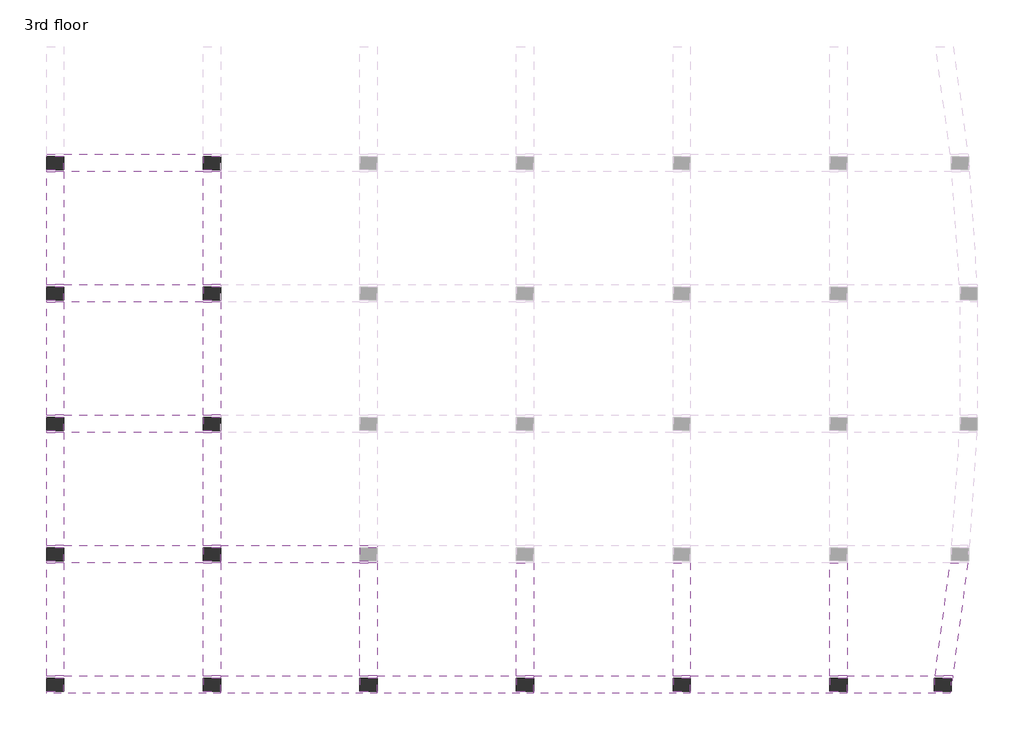
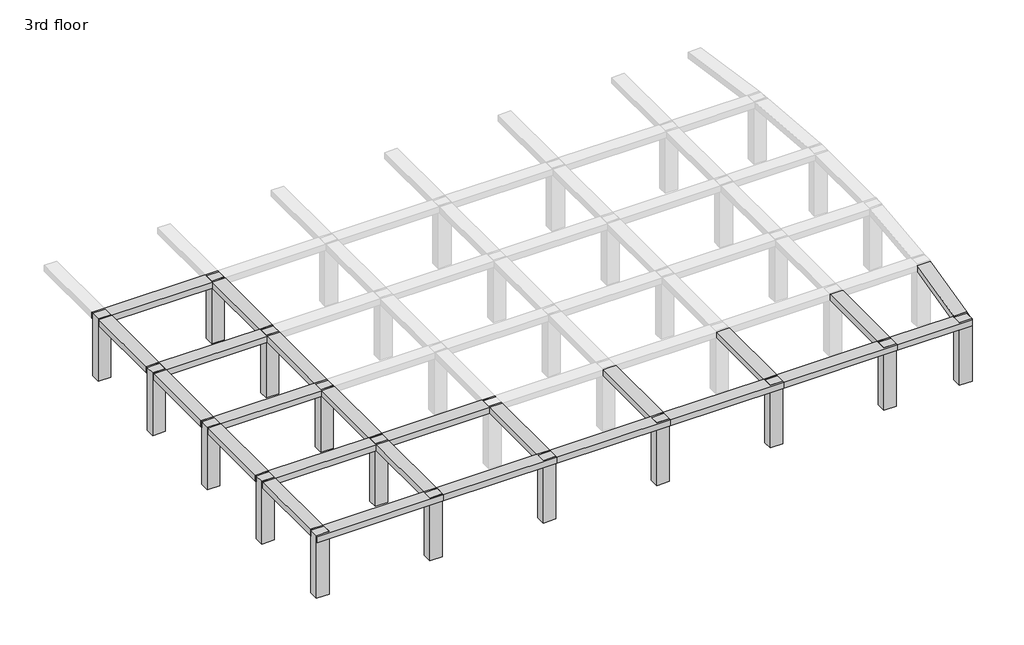
# One storey, part 1 of 3: 24 beams, 15 columns.
"""IFC4 building model written with IfcOpenShell, lengths in millimetres."""

from ifc_helpers import new_model, si_unit, frame, origin, place, context, project, spatial, polyline, outline, extrude, faceted_brep, element, save

model = new_model("IFC4")

# Units and contexts
model_context = context("Model", 3, world=origin())
ifc_project = project(units=[si_unit("LENGTHUNIT", "METRE", prefix="MILLI")], contexts=[model_context])

# Site, building, storey
site = spatial("IfcSite", under=ifc_project)
building = spatial("IfcBuilding", under=site)
storey = spatial("IfcBuildingStorey", under=building, Name="3rd floor", Elevation=9601.2)

# Beams
placement = place(None, origin())
element("IfcBeam", 1, ObjectType="Concrete-Rectangular Beam : 2' x2'", at=placement, inside=storey, context=model_context, shape_type="Brep", body=[
    faceted_brep([(-16619.274232, -2891.2168778, 12801.6), (-17228.874232, -2891.2168778, 12801.6), (-22105.674232, -2891.2168778, 12801.6), (-22715.274232, -2891.2168778, 12801.6), (-22715.274232, -2967.4168778, 12801.6), (-22105.674232, -2967.4168778, 12801.6), (-22105.674232, -3424.6168778, 12801.6), (-22715.274232, -3424.6168778, 12801.6), (-22715.274232, -3500.8168778, 12801.6), (-16619.274232, -3500.8168778, 12801.6), (-16619.274232, -3424.6168778, 12801.6), (-17228.874232, -3424.6168778, 12801.6), (-17228.874232, -2967.4168778, 12801.6), (-16619.274232, -2967.4168778, 12801.6), (-22715.274232, -3500.8168778, 12496.8), (-16619.274232, -3500.8168778, 12496.8), (-22715.274232, -3424.6168778, 12496.8), (-22105.674232, -3424.6168778, 12496.8), (-22105.674232, -2967.4168778, 12496.8), (-22715.274232, -2967.4168778, 12496.8), (-22715.274232, -2891.2168778, 12496.8), (-22105.674232, -2891.2168778, 12496.8), (-17228.874232, -2891.2168778, 12496.8), (-16619.274232, -2891.2168778, 12496.8), (-16619.274232, -2967.4168778, 12496.8), (-17228.874232, -2967.4168778, 12496.8), (-17228.874232, -3424.6168778, 12496.8), (-16619.274232, -3424.6168778, 12496.8)], [[[0, 1, 2, 3, 4, 5, 6, 7, 8, 9, 10, 11, 12, 13]], [[8, 14, 15, 9]], [[15, 14, 16, 17, 18, 19, 20, 21, 22, 23, 24, 25, 26, 27]], [[20, 3, 2, 1, 0, 23, 22, 21]], [[14, 8, 7, 16]], [[9, 15, 27, 10]], [[17, 6, 5, 18]], [[6, 17, 16, 7]], [[18, 5, 4, 19]], [[3, 20, 19, 4]], [[26, 11, 10, 27]], [[11, 26, 25, 12]], [[12, 25, 24, 13]], [[23, 0, 13, 24]]]),
])
element("IfcBeam", 2, ObjectType="Concrete-Rectangular Beam : 2' x2'", at=placement, inside=storey, context=model_context, shape_type="Brep", body=[
    faceted_brep([(-16619.274232, -2891.2168778, 12801.6), (-16619.274232, -2967.4168778, 12801.6), (-16619.274232, -3424.6168778, 12801.6), (-16619.274232, -3500.8168778, 12801.6), (-11132.874232, -3500.8168778, 12801.6), (-11132.874232, -3424.6168778, 12801.6), (-11742.474232, -3424.6168778, 12801.6), (-11742.474232, -2967.4168778, 12801.6), (-11132.874232, -2967.4168778, 12801.6), (-11132.874232, -2891.2168778, 12801.6), (-11742.474232, -2891.2168778, 12801.6), (-11132.874232, -3500.8168778, 12496.8), (-16619.274232, -3500.8168778, 12496.8), (-16619.274232, -3424.6168778, 12496.8), (-16619.274232, -2967.4168778, 12496.8), (-16619.274232, -2891.2168778, 12496.8), (-11742.474232, -2891.2168778, 12496.8), (-11132.874232, -2891.2168778, 12496.8), (-11132.874232, -2967.4168778, 12496.8), (-11742.474232, -2967.4168778, 12496.8), (-11742.474232, -3424.6168778, 12496.8), (-11132.874232, -3424.6168778, 12496.8)], [[[0, 1, 2, 3, 4, 5, 6, 7, 8, 9, 10]], [[11, 4, 3, 12]], [[12, 13, 14, 15, 16, 17, 18, 19, 20, 21, 11]], [[15, 0, 10, 9, 17, 16]], [[3, 2, 1, 0, 15, 14, 13, 12]], [[4, 11, 21, 5]], [[20, 6, 5, 21]], [[6, 20, 19, 7]], [[7, 19, 18, 8]], [[17, 9, 8, 18]]]),
])
element("IfcBeam", 3, ObjectType="Concrete-Rectangular Beam : 2' x2'", at=placement, inside=storey, context=model_context, shape_type="Brep", body=[
    faceted_brep([(-5646.474232, -2891.2168778, 12801.6), (-6256.074232, -2891.2168778, 12801.6), (-11132.874232, -2891.2168778, 12801.6), (-11132.874232, -2967.4168778, 12801.6), (-11132.874232, -3424.6168778, 12801.6), (-11132.874232, -3500.8168778, 12801.6), (-5646.474232, -3500.8168778, 12801.6), (-5646.474232, -3424.6168778, 12801.6), (-6256.074232, -3424.6168778, 12801.6), (-6256.074232, -2967.4168778, 12801.6), (-5646.474232, -2967.4168778, 12801.6), (-5646.474232, -3500.8168778, 12496.8), (-11132.874232, -3500.8168778, 12496.8), (-11132.874232, -3424.6168778, 12496.8), (-11132.874232, -2967.4168778, 12496.8), (-11132.874232, -2891.2168778, 12496.8), (-6256.074232, -2891.2168778, 12496.8), (-5646.474232, -2891.2168778, 12496.8), (-5646.474232, -2967.4168778, 12496.8), (-6256.074232, -2967.4168778, 12496.8), (-6256.074232, -3424.6168778, 12496.8), (-5646.474232, -3424.6168778, 12496.8)], [[[0, 1, 2, 3, 4, 5, 6, 7, 8, 9, 10]], [[11, 6, 5, 12]], [[11, 12, 13, 14, 15, 16, 17, 18, 19, 20, 21]], [[0, 17, 16, 15, 2, 1]], [[6, 11, 21, 7]], [[5, 4, 3, 2, 15, 14, 13, 12]], [[20, 8, 7, 21]], [[8, 20, 19, 9]], [[9, 19, 18, 10]], [[17, 0, 10, 18]]]),
])
element("IfcBeam", 4, ObjectType="Concrete-Rectangular Beam : 2' x2'", at=placement, inside=storey, context=model_context, shape_type="Brep", body=[
    faceted_brep([(-5646.474232, -2891.2168778, 12801.6), (-5646.474232, -2967.4168778, 12801.6), (-5646.474232, -3424.6168778, 12801.6), (-5646.474232, -3500.8168778, 12801.6), (-160.074232, -3500.8168778, 12801.6), (-160.074232, -3424.6168778, 12801.6), (-769.674232, -3424.6168778, 12801.6), (-769.674232, -2967.4168778, 12801.6), (-160.074232, -2967.4168778, 12801.6), (-160.074232, -2891.2168778, 12801.6), (-769.674232, -2891.2168778, 12801.6), (-160.074232, -3500.8168778, 12496.8), (-5646.474232, -3500.8168778, 12496.8), (-5646.474232, -3424.6168778, 12496.8), (-5646.474232, -2967.4168778, 12496.8), (-5646.474232, -2891.2168778, 12496.8), (-769.674232, -2891.2168778, 12496.8), (-160.074232, -2891.2168778, 12496.8), (-160.074232, -2967.4168778, 12496.8), (-769.674232, -2967.4168778, 12496.8), (-769.674232, -3424.6168778, 12496.8), (-160.074232, -3424.6168778, 12496.8)], [[[0, 1, 2, 3, 4, 5, 6, 7, 8, 9, 10]], [[11, 4, 3, 12]], [[12, 13, 14, 15, 16, 17, 18, 19, 20, 21, 11]], [[15, 0, 10, 9, 17, 16]], [[3, 2, 1, 0, 15, 14, 13, 12]], [[4, 11, 21, 5]], [[20, 6, 5, 21]], [[6, 20, 19, 7]], [[7, 19, 18, 8]], [[17, 9, 8, 18]]]),
])
element("IfcBeam", 5, ObjectType="Concrete-Rectangular Beam : 2' x2'", at=placement, inside=storey, context=model_context, shape_type="Brep", body=[
    faceted_brep([(-160.074232, -2891.2168778, 12801.6), (-160.074232, -2967.4168778, 12801.6), (-160.074232, -3424.6168778, 12801.6), (-160.074232, -3500.8168778, 12801.6), (5326.325768, -3500.8168778, 12801.6), (5326.325768, -3424.6168778, 12801.6), (4716.725768, -3424.6168778, 12801.6), (4716.725768, -2967.4168778, 12801.6), (5326.325768, -2967.4168778, 12801.6), (5326.325768, -2891.2168778, 12801.6), (4716.725768, -2891.2168778, 12801.6), (5326.325768, -3500.8168778, 12496.8), (-160.074232, -3500.8168778, 12496.8), (-160.074232, -3424.6168778, 12496.8), (-160.074232, -2967.4168778, 12496.8), (-160.074232, -2891.2168778, 12496.8), (4716.725768, -2891.2168778, 12496.8), (5326.325768, -2891.2168778, 12496.8), (5326.325768, -2967.4168778, 12496.8), (4716.725768, -2967.4168778, 12496.8), (4716.725768, -3424.6168778, 12496.8), (5326.325768, -3424.6168778, 12496.8)], [[[0, 1, 2, 3, 4, 5, 6, 7, 8, 9, 10]], [[11, 4, 3, 12]], [[12, 13, 14, 15, 16, 17, 18, 19, 20, 21, 11]], [[15, 0, 10, 9, 17, 16]], [[3, 2, 1, 0, 15, 14, 13, 12]], [[4, 11, 21, 5]], [[20, 6, 5, 21]], [[6, 20, 19, 7]], [[7, 19, 18, 8]], [[17, 9, 8, 18]]]),
])
element("IfcBeam", 6, ObjectType="Concrete-Rectangular Beam : 2' x2'", at=placement, inside=storey, context=model_context, shape_type="Brep", body=[
    faceted_brep([(9027.2344863, -2891.2168778, 12801.6), (8412.2463849, -2891.2168778, 12801.6), (5326.325768, -2891.2168778, 12801.6), (5326.325768, -2967.4168778, 12801.6), (5326.325768, -3424.6168778, 12801.6), (5326.325768, -3500.8168778, 12801.6), (8946.005151, -3500.8168778, 12801.6), (8956.158818, -3424.6168778, 12801.6), (8374.325768, -3424.6168778, 12801.6), (8374.325768, -2967.4168778, 12801.6), (8983.925768, -2967.4168778, 12801.6), (8983.925768, -3216.2348608, 12801.6), (8946.005151, -3500.8168778, 12496.8), (5326.325768, -3500.8168778, 12496.8), (5326.325768, -3424.6168778, 12496.8), (5326.325768, -2967.4168778, 12496.8), (5326.325768, -2891.2168778, 12496.8), (8412.2463849, -2891.2168778, 12496.8), (9027.2344863, -2891.2168778, 12496.8), (8983.925768, -3216.2348608, 12496.8), (8983.925768, -2967.4168778, 12496.8), (8374.325768, -2967.4168778, 12496.8), (8374.325768, -3424.6168778, 12496.8), (8956.158818, -3424.6168778, 12496.8)], [[[0, 1, 2, 3, 4, 5, 6, 7, 8, 9, 10, 11]], [[12, 6, 5, 13]], [[12, 13, 14, 15, 16, 17, 18, 19, 20, 21, 22, 23]], [[0, 18, 17, 16, 2, 1]], [[6, 12, 23, 7]], [[5, 4, 3, 2, 16, 15, 14, 13]], [[10, 20, 19, 11]], [[22, 8, 7, 23]], [[8, 22, 21, 9]], [[9, 21, 20, 10]], [[18, 0, 11, 19]]]),
])
element("IfcBeam", 7, ObjectType="Concrete-Rectangular Beam : 2' x2'", at=placement, inside=storey, context=model_context, shape_type="Brep", body=[
    faceted_brep([(-16619.274232, 1680.7831222, 12801.6), (-17228.874232, 1680.7831222, 12801.6), (-22105.674232, 1680.7831222, 12801.6), (-22715.274232, 1680.7831222, 12801.6), (-22715.274232, 1604.5831222, 12801.6), (-22105.674232, 1604.5831222, 12801.6), (-22105.674232, 1147.3831222, 12801.6), (-22715.274232, 1147.3831222, 12801.6), (-22715.274232, 1071.1831222, 12801.6), (-22105.674232, 1071.1831222, 12801.6), (-17228.874232, 1071.1831222, 12801.6), (-16619.274232, 1071.1831222, 12801.6), (-16619.274232, 1147.3831222, 12801.6), (-17228.874232, 1147.3831222, 12801.6), (-17228.874232, 1604.5831222, 12801.6), (-16619.274232, 1604.5831222, 12801.6), (-22715.274232, 1071.1831222, 12496.8), (-22105.674232, 1071.1831222, 12496.8), (-17228.874232, 1071.1831222, 12496.8), (-16619.274232, 1071.1831222, 12496.8), (-22715.274232, 1147.3831222, 12496.8), (-22105.674232, 1147.3831222, 12496.8), (-22105.674232, 1604.5831222, 12496.8), (-22715.274232, 1604.5831222, 12496.8), (-22715.274232, 1680.7831222, 12496.8), (-22105.674232, 1680.7831222, 12496.8), (-17228.874232, 1680.7831222, 12496.8), (-16619.274232, 1680.7831222, 12496.8), (-16619.274232, 1604.5831222, 12496.8), (-17228.874232, 1604.5831222, 12496.8), (-17228.874232, 1147.3831222, 12496.8), (-16619.274232, 1147.3831222, 12496.8)], [[[0, 1, 2, 3, 4, 5, 6, 7, 8, 9, 10, 11, 12, 13, 14, 15]], [[8, 16, 17, 18, 19, 11, 10, 9]], [[19, 18, 17, 16, 20, 21, 22, 23, 24, 25, 26, 27, 28, 29, 30, 31]], [[24, 3, 2, 1, 0, 27, 26, 25]], [[16, 8, 7, 20]], [[11, 19, 31, 12]], [[21, 6, 5, 22]], [[6, 21, 20, 7]], [[22, 5, 4, 23]], [[3, 24, 23, 4]], [[30, 13, 12, 31]], [[13, 30, 29, 14]], [[14, 29, 28, 15]], [[27, 0, 15, 28]]]),
])
element("IfcBeam", 8, ObjectType="Concrete-Rectangular Beam : 2' x2'", at=placement, inside=storey, context=model_context, shape_type="Brep", body=[
    faceted_brep([(-16619.274232, 1680.7831222, 12801.6), (-16619.274232, 1604.5831222, 12801.6), (-16619.274232, 1147.3831222, 12801.6), (-16619.274232, 1071.1831222, 12801.6), (-11742.474232, 1071.1831222, 12801.6), (-11132.874232, 1071.1831222, 12801.6), (-11132.874232, 1147.3831222, 12801.6), (-11742.474232, 1147.3831222, 12801.6), (-11742.474232, 1604.5831222, 12801.6), (-11132.874232, 1604.5831222, 12801.6), (-11132.874232, 1680.7831222, 12801.6), (-11742.474232, 1680.7831222, 12801.6), (-16619.274232, 1071.1831222, 12496.8), (-11742.474232, 1071.1831222, 12496.8), (-11132.874232, 1071.1831222, 12496.8), (-16619.274232, 1147.3831222, 12496.8), (-16619.274232, 1604.5831222, 12496.8), (-16619.274232, 1680.7831222, 12496.8), (-11742.474232, 1680.7831222, 12496.8), (-11132.874232, 1680.7831222, 12496.8), (-11132.874232, 1604.5831222, 12496.8), (-11742.474232, 1604.5831222, 12496.8), (-11742.474232, 1147.3831222, 12496.8), (-11132.874232, 1147.3831222, 12496.8)], [[[0, 1, 2, 3, 4, 5, 6, 7, 8, 9, 10, 11]], [[3, 12, 13, 14, 5, 4]], [[12, 15, 16, 17, 18, 19, 20, 21, 22, 23, 14, 13]], [[10, 19, 18, 17, 0, 11]], [[3, 2, 1, 0, 17, 16, 15, 12]], [[5, 14, 23, 6]], [[22, 7, 6, 23]], [[7, 22, 21, 8]], [[8, 21, 20, 9]], [[19, 10, 9, 20]]]),
])
element("IfcBeam", 9, ObjectType="Concrete-Rectangular Beam : 2' x2'", at=placement, inside=storey, context=model_context, shape_type="Brep", body=[
    faceted_brep([(-16619.274232, 6252.7831222, 12801.6), (-17228.874232, 6252.7831222, 12801.6), (-22105.674232, 6252.7831222, 12801.6), (-22715.274232, 6252.7831222, 12801.6), (-22715.274232, 6176.5831222, 12801.6), (-22105.674232, 6176.5831222, 12801.6), (-22105.674232, 5719.3831222, 12801.6), (-22715.274232, 5719.3831222, 12801.6), (-22715.274232, 5643.1831222, 12801.6), (-22105.674232, 5643.1831222, 12801.6), (-17228.874232, 5643.1831222, 12801.6), (-16619.274232, 5643.1831222, 12801.6), (-16619.274232, 5719.3831222, 12801.6), (-17228.874232, 5719.3831222, 12801.6), (-17228.874232, 6176.5831222, 12801.6), (-16619.274232, 6176.5831222, 12801.6), (-22715.274232, 5643.1831222, 12496.8), (-22105.674232, 5643.1831222, 12496.8), (-17228.874232, 5643.1831222, 12496.8), (-16619.274232, 5643.1831222, 12496.8), (-22715.274232, 5719.3831222, 12496.8), (-22105.674232, 5719.3831222, 12496.8), (-22105.674232, 6176.5831222, 12496.8), (-22715.274232, 6176.5831222, 12496.8), (-22715.274232, 6252.7831222, 12496.8), (-22105.674232, 6252.7831222, 12496.8), (-17228.874232, 6252.7831222, 12496.8), (-16619.274232, 6252.7831222, 12496.8), (-16619.274232, 6176.5831222, 12496.8), (-17228.874232, 6176.5831222, 12496.8), (-17228.874232, 5719.3831222, 12496.8), (-16619.274232, 5719.3831222, 12496.8)], [[[0, 1, 2, 3, 4, 5, 6, 7, 8, 9, 10, 11, 12, 13, 14, 15]], [[8, 16, 17, 18, 19, 11, 10, 9]], [[19, 18, 17, 16, 20, 21, 22, 23, 24, 25, 26, 27, 28, 29, 30, 31]], [[24, 3, 2, 1, 0, 27, 26, 25]], [[16, 8, 7, 20]], [[11, 19, 31, 12]], [[21, 6, 5, 22]], [[6, 21, 20, 7]], [[22, 5, 4, 23]], [[3, 24, 23, 4]], [[30, 13, 12, 31]], [[13, 30, 29, 14]], [[14, 29, 28, 15]], [[27, 0, 15, 28]]]),
])
element("IfcBeam", 10, ObjectType="Concrete-Rectangular Beam : 2' x2'", at=placement, inside=storey, context=model_context, shape_type="Brep", body=[
    faceted_brep([(-16619.274232, 10824.7831222, 12801.6), (-17228.874232, 10824.7831222, 12801.6), (-22105.674232, 10824.7831222, 12801.6), (-22715.274232, 10824.7831222, 12801.6), (-22715.274232, 10748.5831222, 12801.6), (-22105.674232, 10748.5831222, 12801.6), (-22105.674232, 10291.3831222, 12801.6), (-22715.274232, 10291.3831222, 12801.6), (-22715.274232, 10215.1831222, 12801.6), (-22105.674232, 10215.1831222, 12801.6), (-17228.874232, 10215.1831222, 12801.6), (-16619.274232, 10215.1831222, 12801.6), (-16619.274232, 10291.3831222, 12801.6), (-17228.874232, 10291.3831222, 12801.6), (-17228.874232, 10748.5831222, 12801.6), (-16619.274232, 10748.5831222, 12801.6), (-22715.274232, 10215.1831222, 12496.8), (-22105.674232, 10215.1831222, 12496.8), (-17228.874232, 10215.1831222, 12496.8), (-16619.274232, 10215.1831222, 12496.8), (-22715.274232, 10291.3831222, 12496.8), (-22105.674232, 10291.3831222, 12496.8), (-22105.674232, 10748.5831222, 12496.8), (-22715.274232, 10748.5831222, 12496.8), (-22715.274232, 10824.7831222, 12496.8), (-22105.674232, 10824.7831222, 12496.8), (-17228.874232, 10824.7831222, 12496.8), (-16619.274232, 10824.7831222, 12496.8), (-16619.274232, 10748.5831222, 12496.8), (-17228.874232, 10748.5831222, 12496.8), (-17228.874232, 10291.3831222, 12496.8), (-16619.274232, 10291.3831222, 12496.8)], [[[0, 1, 2, 3, 4, 5, 6, 7, 8, 9, 10, 11, 12, 13, 14, 15]], [[8, 16, 17, 18, 19, 11, 10, 9]], [[19, 18, 17, 16, 20, 21, 22, 23, 24, 25, 26, 27, 28, 29, 30, 31]], [[24, 3, 2, 1, 0, 27, 26, 25]], [[16, 8, 7, 20]], [[11, 19, 31, 12]], [[21, 6, 5, 22]], [[6, 21, 20, 7]], [[22, 5, 4, 23]], [[3, 24, 23, 4]], [[30, 13, 12, 31]], [[13, 30, 29, 14]], [[14, 29, 28, 15]], [[27, 0, 15, 28]]]),
])
element("IfcBeam", 11, ObjectType="Concrete-Rectangular Beam : 2' x2'", at=placement, inside=storey, context=model_context, shape_type="Brep", body=[
    faceted_brep([(-16619.274232, 15396.7831222, 12801.6), (-17228.874232, 15396.7831222, 12801.6), (-22105.674232, 15396.7831222, 12801.6), (-22715.274232, 15396.7831222, 12801.6), (-22715.274232, 15320.5831222, 12801.6), (-22105.674232, 15320.5831222, 12801.6), (-22105.674232, 14863.3831222, 12801.6), (-22715.274232, 14863.3831222, 12801.6), (-22715.274232, 14787.1831222, 12801.6), (-22105.674232, 14787.1831222, 12801.6), (-17228.874232, 14787.1831222, 12801.6), (-16619.274232, 14787.1831222, 12801.6), (-16619.274232, 14863.3831222, 12801.6), (-17228.874232, 14863.3831222, 12801.6), (-17228.874232, 15320.5831222, 12801.6), (-16619.274232, 15320.5831222, 12801.6), (-22715.274232, 14787.1831222, 12496.8), (-22105.674232, 14787.1831222, 12496.8), (-17228.874232, 14787.1831222, 12496.8), (-16619.274232, 14787.1831222, 12496.8), (-22715.274232, 14863.3831222, 12496.8), (-22105.674232, 14863.3831222, 12496.8), (-22105.674232, 15320.5831222, 12496.8), (-22715.274232, 15320.5831222, 12496.8), (-22715.274232, 15396.7831222, 12496.8), (-22105.674232, 15396.7831222, 12496.8), (-17228.874232, 15396.7831222, 12496.8), (-16619.274232, 15396.7831222, 12496.8), (-16619.274232, 15320.5831222, 12496.8), (-17228.874232, 15320.5831222, 12496.8), (-17228.874232, 14863.3831222, 12496.8), (-16619.274232, 14863.3831222, 12496.8)], [[[0, 1, 2, 3, 4, 5, 6, 7, 8, 9, 10, 11, 12, 13, 14, 15]], [[8, 16, 17, 18, 19, 11, 10, 9]], [[19, 18, 17, 16, 20, 21, 22, 23, 24, 25, 26, 27, 28, 29, 30, 31]], [[24, 3, 2, 1, 0, 27, 26, 25]], [[16, 8, 7, 20]], [[11, 19, 31, 12]], [[21, 6, 5, 22]], [[6, 21, 20, 7]], [[22, 5, 4, 23]], [[3, 24, 23, 4]], [[30, 13, 12, 31]], [[13, 30, 29, 14]], [[14, 29, 28, 15]], [[27, 0, 15, 28]]]),
])
element("IfcBeam", 12, ObjectType="Concrete-Rectangular Beam : 2' x2'", at=placement, inside=storey, context=model_context, shape_type="SweptSolid", body=[
    extrude(outline(polyline([(-22105.674232, -2891.2168778), (-22715.274232, -2891.2168778), (-22715.274232, 1071.1831222), (-22105.674232, 1071.1831222), (-22105.674232, -2891.2168778)])), frame((0.0, 0.0, 12496.8), z_axis=(0.0, 0.0, 1.0), x_axis=(1.0, 0.0, 0.0)), (0.0, 0.0, 1.0), 304.8),
])
element("IfcBeam", 13, ObjectType="Concrete-Rectangular Beam : 2' x2'", at=placement, inside=storey, context=model_context, shape_type="SweptSolid", body=[
    extrude(outline(polyline([(-22105.674232, 1680.7831222), (-22715.274232, 1680.7831222), (-22715.274232, 5643.1831222), (-22105.674232, 5643.1831222), (-22105.674232, 1680.7831222)])), frame((0.0, 0.0, 12496.8), z_axis=(0.0, 0.0, 1.0), x_axis=(1.0, 0.0, 0.0)), (0.0, 0.0, 1.0), 304.8),
])
element("IfcBeam", 14, ObjectType="Concrete-Rectangular Beam : 2' x2'", at=placement, inside=storey, context=model_context, shape_type="SweptSolid", body=[
    extrude(outline(polyline([(-22105.674232, 6252.7831222), (-22715.274232, 6252.7831222), (-22715.274232, 10215.1831222), (-22105.674232, 10215.1831222), (-22105.674232, 6252.7831222)])), frame((0.0, 0.0, 12496.8), z_axis=(0.0, 0.0, 1.0), x_axis=(1.0, 0.0, 0.0)), (0.0, 0.0, 1.0), 304.8),
])
element("IfcBeam", 15, ObjectType="Concrete-Rectangular Beam : 2' x2'", at=placement, inside=storey, context=model_context, shape_type="SweptSolid", body=[
    extrude(outline(polyline([(-22105.674232, 10824.7831222), (-22715.274232, 10824.7831222), (-22715.274232, 14787.1831222), (-22105.674232, 14787.1831222), (-22105.674232, 10824.7831222)])), frame((0.0, 0.0, 12496.8), z_axis=(0.0, 0.0, 1.0), x_axis=(1.0, 0.0, 0.0)), (0.0, 0.0, 1.0), 304.8),
])
element("IfcBeam", 16, ObjectType="Concrete-Rectangular Beam : 2' x2'", at=placement, inside=storey, context=model_context, shape_type="SweptSolid", body=[
    extrude(outline(polyline([(-17228.874232, 1071.1831222), (-16619.274232, 1071.1831222), (-16619.274232, -2891.2168778), (-17228.874232, -2891.2168778), (-17228.874232, 1071.1831222)])), frame((0.0, 0.0, 12496.8), z_axis=(0.0, 0.0, 1.0), x_axis=(1.0, 0.0, 0.0)), (0.0, 0.0, 1.0), 304.8),
])
element("IfcBeam", 17, ObjectType="Concrete-Rectangular Beam : 2' x2'", at=placement, inside=storey, context=model_context, shape_type="SweptSolid", body=[
    extrude(outline(polyline([(-16619.274232, 1680.7831222), (-17228.874232, 1680.7831222), (-17228.874232, 5643.1831222), (-16619.274232, 5643.1831222), (-16619.274232, 1680.7831222)])), frame((0.0, 0.0, 12496.8), z_axis=(0.0, 0.0, 1.0), x_axis=(1.0, 0.0, 0.0)), (0.0, 0.0, 1.0), 304.8),
])
element("IfcBeam", 18, ObjectType="Concrete-Rectangular Beam : 2' x2'", at=placement, inside=storey, context=model_context, shape_type="SweptSolid", body=[
    extrude(outline(polyline([(-16619.274232, 6252.7831222), (-17228.874232, 6252.7831222), (-17228.874232, 10215.1831222), (-16619.274232, 10215.1831222), (-16619.274232, 6252.7831222)])), frame((0.0, 0.0, 12496.8), z_axis=(0.0, 0.0, 1.0), x_axis=(1.0, 0.0, 0.0)), (0.0, 0.0, 1.0), 304.8),
])
element("IfcBeam", 19, ObjectType="Concrete-Rectangular Beam : 2' x2'", at=placement, inside=storey, context=model_context, shape_type="SweptSolid", body=[
    extrude(outline(polyline([(-16619.274232, 10824.7831222), (-17228.874232, 10824.7831222), (-17228.874232, 14787.1831222), (-16619.274232, 14787.1831222), (-16619.274232, 10824.7831222)])), frame((0.0, 0.0, 12496.8), z_axis=(0.0, 0.0, 1.0), x_axis=(1.0, 0.0, 0.0)), (0.0, 0.0, 1.0), 304.8),
])
element("IfcBeam", 20, ObjectType="Concrete-Rectangular Beam : 2' x2'", at=placement, inside=storey, context=model_context, shape_type="SweptSolid", body=[
    extrude(outline(polyline([(-11742.474232, 1071.1831222), (-11132.874232, 1071.1831222), (-11132.874232, -2891.2168778), (-11742.474232, -2891.2168778), (-11742.474232, 1071.1831222)])), frame((0.0, 0.0, 12496.8), z_axis=(0.0, 0.0, 1.0), x_axis=(1.0, 0.0, 0.0)), (0.0, 0.0, 1.0), 304.8),
])
element("IfcBeam", 21, ObjectType="Concrete-Rectangular Beam : 2' x2'", at=placement, inside=storey, context=model_context, shape_type="SweptSolid", body=[
    extrude(outline(polyline([(-6256.074232, 1071.1831222), (-5646.474232, 1071.1831222), (-5646.474232, -2891.2168778), (-6256.074232, -2891.2168778), (-6256.074232, 1071.1831222)])), frame((0.0, 0.0, 12496.8), z_axis=(0.0, 0.0, 1.0), x_axis=(1.0, 0.0, 0.0)), (0.0, 0.0, 1.0), 304.8),
])
element("IfcBeam", 22, ObjectType="Concrete-Rectangular Beam : 2' x2'", at=placement, inside=storey, context=model_context, shape_type="SweptSolid", body=[
    extrude(outline(polyline([(-769.674232, 1071.1831222), (-160.074232, 1071.1831222), (-160.074232, -2891.2168778), (-769.674232, -2891.2168778), (-769.674232, 1071.1831222)])), frame((0.0, 0.0, 12496.8), z_axis=(0.0, 0.0, 1.0), x_axis=(1.0, 0.0, 0.0)), (0.0, 0.0, 1.0), 304.8),
])
element("IfcBeam", 23, ObjectType="Concrete-Rectangular Beam : 2' x2'", at=placement, inside=storey, context=model_context, shape_type="SweptSolid", body=[
    extrude(outline(polyline([(4716.725768, 1071.1831222), (5326.325768, 1071.1831222), (5326.325768, -2891.2168778), (4716.725768, -2891.2168778), (4716.725768, 1071.1831222)])), frame((0.0, 0.0, 12496.8), z_axis=(0.0, 0.0, 1.0), x_axis=(1.0, 0.0, 0.0)), (0.0, 0.0, 1.0), 304.8),
])
element("IfcBeam", 24, ObjectType="Concrete-Rectangular Beam : 2' x2'", at=placement, inside=storey, context=model_context, shape_type="SweptSolid", body=[
    extrude(outline(polyline([(8940.2370643, 1071.1831222), (9555.2251658, 1071.1831222), (9027.2344863, -2891.2168778), (8412.2463849, -2891.2168778), (8940.2370643, 1071.1831222)])), frame((0.0, 0.0, 12496.8), z_axis=(0.0, 0.0, 1.0), x_axis=(1.0, 0.0, 0.0)), (0.0, 0.0, 1.0), 304.8),
])

# Columns
element("IfcColumn", 25, ObjectType="Concrete-Rectangular-Column : 12 x 18", at=placement, inside=storey, context=model_context, shape_type="SweptSolid", body=[
    extrude(outline(polyline([(-22105.674232, -2967.4168778), (-22105.674232, -3424.6168778), (-22715.274232, -3424.6168778), (-22715.274232, -2967.4168778), (-22105.674232, -2967.4168778)])), frame((0.0, 0.0, 9601.2), z_axis=(0.0, 0.0, 1.0), x_axis=(1.0, 0.0, 0.0)), (0.0, 0.0, 1.0), 3200.4),
])
element("IfcColumn", 26, ObjectType="Concrete-Rectangular-Column : 12 x 18", at=placement, inside=storey, context=model_context, shape_type="SweptSolid", body=[
    extrude(outline(polyline([(-16619.274232, -2967.4168778), (-16619.274232, -3424.6168778), (-17228.874232, -3424.6168778), (-17228.874232, -2967.4168778), (-16619.274232, -2967.4168778)])), frame((0.0, 0.0, 9601.2), z_axis=(0.0, 0.0, 1.0), x_axis=(1.0, 0.0, 0.0)), (0.0, 0.0, 1.0), 3200.4),
])
element("IfcColumn", 27, ObjectType="Concrete-Rectangular-Column : 12 x 18", at=placement, inside=storey, context=model_context, shape_type="SweptSolid", body=[
    extrude(outline(polyline([(-11132.874232, -2967.4168778), (-11132.874232, -3424.6168778), (-11742.474232, -3424.6168778), (-11742.474232, -2967.4168778), (-11132.874232, -2967.4168778)])), frame((0.0, 0.0, 9601.2), z_axis=(0.0, 0.0, 1.0), x_axis=(1.0, 0.0, 0.0)), (0.0, 0.0, 1.0), 3200.4),
])
element("IfcColumn", 28, ObjectType="Concrete-Rectangular-Column : 12 x 18", at=placement, inside=storey, context=model_context, shape_type="SweptSolid", body=[
    extrude(outline(polyline([(-5646.474232, -2967.4168778), (-5646.474232, -3424.6168778), (-6256.074232, -3424.6168778), (-6256.074232, -2967.4168778), (-5646.474232, -2967.4168778)])), frame((0.0, 0.0, 9601.2), z_axis=(0.0, 0.0, 1.0), x_axis=(1.0, 0.0, 0.0)), (0.0, 0.0, 1.0), 3200.4),
])
element("IfcColumn", 29, ObjectType="Concrete-Rectangular-Column : 12 x 18", at=placement, inside=storey, context=model_context, shape_type="SweptSolid", body=[
    extrude(outline(polyline([(-160.074232, -2967.4168778), (-160.074232, -3424.6168778), (-769.674232, -3424.6168778), (-769.674232, -2967.4168778), (-160.074232, -2967.4168778)])), frame((0.0, 0.0, 9601.2), z_axis=(0.0, 0.0, 1.0), x_axis=(1.0, 0.0, 0.0)), (0.0, 0.0, 1.0), 3200.4),
])
element("IfcColumn", 30, ObjectType="Concrete-Rectangular-Column : 12 x 18", at=placement, inside=storey, context=model_context, shape_type="SweptSolid", body=[
    extrude(outline(polyline([(5326.325768, -2967.4168778), (5326.325768, -3424.6168778), (4716.725768, -3424.6168778), (4716.725768, -2967.4168778), (5326.325768, -2967.4168778)])), frame((0.0, 0.0, 9601.2), z_axis=(0.0, 0.0, 1.0), x_axis=(1.0, 0.0, 0.0)), (0.0, 0.0, 1.0), 3200.4),
])
element("IfcColumn", 31, ObjectType="Concrete-Rectangular-Column : 12 x 18", at=placement, inside=storey, context=model_context, shape_type="SweptSolid", body=[
    extrude(outline(polyline([(8983.925768, -2967.4168778), (8983.925768, -3424.6168778), (8374.325768, -3424.6168778), (8374.325768, -2967.4168778), (8983.925768, -2967.4168778)])), frame((0.0, 0.0, 9601.2), z_axis=(0.0, 0.0, 1.0), x_axis=(1.0, 0.0, 0.0)), (0.0, 0.0, 1.0), 3200.4),
])
element("IfcColumn", 32, ObjectType="Concrete-Rectangular-Column : 12 x 18", at=placement, inside=storey, context=model_context, shape_type="SweptSolid", body=[
    extrude(outline(polyline([(-22105.674232, 1604.5831222), (-22105.674232, 1147.3831222), (-22715.274232, 1147.3831222), (-22715.274232, 1604.5831222), (-22105.674232, 1604.5831222)])), frame((0.0, 0.0, 9601.2), z_axis=(0.0, 0.0, 1.0), x_axis=(1.0, 0.0, 0.0)), (0.0, 0.0, 1.0), 3200.4),
])
element("IfcColumn", 33, ObjectType="Concrete-Rectangular-Column : 12 x 18", at=placement, inside=storey, context=model_context, shape_type="SweptSolid", body=[
    extrude(outline(polyline([(-16619.274232, 1604.5831222), (-16619.274232, 1147.3831222), (-17228.874232, 1147.3831222), (-17228.874232, 1604.5831222), (-16619.274232, 1604.5831222)])), frame((0.0, 0.0, 9601.2), z_axis=(0.0, 0.0, 1.0), x_axis=(1.0, 0.0, 0.0)), (0.0, 0.0, 1.0), 3200.4),
])
element("IfcColumn", 34, ObjectType="Concrete-Rectangular-Column : 12 x 18", at=placement, inside=storey, context=model_context, shape_type="SweptSolid", body=[
    extrude(outline(polyline([(-22105.674232, 6176.5831222), (-22105.674232, 5719.3831222), (-22715.274232, 5719.3831222), (-22715.274232, 6176.5831222), (-22105.674232, 6176.5831222)])), frame((0.0, 0.0, 9601.2), z_axis=(0.0, 0.0, 1.0), x_axis=(1.0, 0.0, 0.0)), (0.0, 0.0, 1.0), 3200.4),
])
element("IfcColumn", 35, ObjectType="Concrete-Rectangular-Column : 12 x 18", at=placement, inside=storey, context=model_context, shape_type="SweptSolid", body=[
    extrude(outline(polyline([(-16619.274232, 6176.5831222), (-16619.274232, 5719.3831222), (-17228.874232, 5719.3831222), (-17228.874232, 6176.5831222), (-16619.274232, 6176.5831222)])), frame((0.0, 0.0, 9601.2), z_axis=(0.0, 0.0, 1.0), x_axis=(1.0, 0.0, 0.0)), (0.0, 0.0, 1.0), 3200.4),
])
element("IfcColumn", 36, ObjectType="Concrete-Rectangular-Column : 12 x 18", at=placement, inside=storey, context=model_context, shape_type="SweptSolid", body=[
    extrude(outline(polyline([(-22105.674232, 10748.5831222), (-22105.674232, 10291.3831222), (-22715.274232, 10291.3831222), (-22715.274232, 10748.5831222), (-22105.674232, 10748.5831222)])), frame((0.0, 0.0, 9601.2), z_axis=(0.0, 0.0, 1.0), x_axis=(1.0, 0.0, 0.0)), (0.0, 0.0, 1.0), 3200.4),
])
element("IfcColumn", 37, ObjectType="Concrete-Rectangular-Column : 12 x 18", at=placement, inside=storey, context=model_context, shape_type="SweptSolid", body=[
    extrude(outline(polyline([(-16619.274232, 10748.5831222), (-16619.274232, 10291.3831222), (-17228.874232, 10291.3831222), (-17228.874232, 10748.5831222), (-16619.274232, 10748.5831222)])), frame((0.0, 0.0, 9601.2), z_axis=(0.0, 0.0, 1.0), x_axis=(1.0, 0.0, 0.0)), (0.0, 0.0, 1.0), 3200.4),
])
element("IfcColumn", 38, ObjectType="Concrete-Rectangular-Column : 12 x 18", at=placement, inside=storey, context=model_context, shape_type="SweptSolid", body=[
    extrude(outline(polyline([(-22105.674232, 15320.5831222), (-22105.674232, 14863.3831222), (-22715.274232, 14863.3831222), (-22715.274232, 15320.5831222), (-22105.674232, 15320.5831222)])), frame((0.0, 0.0, 9601.2), z_axis=(0.0, 0.0, 1.0), x_axis=(1.0, 0.0, 0.0)), (0.0, 0.0, 1.0), 3200.4),
])
element("IfcColumn", 39, ObjectType="Concrete-Rectangular-Column : 12 x 18", at=placement, inside=storey, context=model_context, shape_type="SweptSolid", body=[
    extrude(outline(polyline([(-16619.274232, 15320.5831222), (-16619.274232, 14863.3831222), (-17228.874232, 14863.3831222), (-17228.874232, 15320.5831222), (-16619.274232, 15320.5831222)])), frame((0.0, 0.0, 9601.2), z_axis=(0.0, 0.0, 1.0), x_axis=(1.0, 0.0, 0.0)), (0.0, 0.0, 1.0), 3200.4),
])

save(model, "model.ifc")

# Revit data of these elements
# Type "Concrete-Rectangular Beam : 2' x2'"
#   Assembly Code = "B10"
#   Length [instance default] = 5' - 0"
#   b = 2' - 0"
#   h = 1' - 0"
#   Structural Material [instance default] = Concrete, Cast-in-Place gray
# Type "Concrete-Rectangular-Column : 12 x 18"
#   Assembly Code = "B10"
#   b = 2' - 0"
#   h = 1' - 6"
#   Structural Material [instance default] = Concrete, Cast-in-Place gray
# Elements 1, 2, 3, 4, 5, 6, 7, 8, 9, 10, 11, 12, 13, 14, 15, 16, 17, 18, 19, 20, 21, 22, 23, 24 (IfcBeam, "Concrete-Rectangular Beam : 2' x2'")
#   Structural Material = Concrete, Precast (2)
#   Phase Created = New Construction
#   Materials on its faces: "Concrete, Precast (2)"
# Elements 25, 26, 27, 28, 29, 30, 31, 32, 33, 34, 35, 36, 37, 38, 39 (IfcColumn, "Concrete-Rectangular-Column : 12 x 18")
#   Phase Created = New Construction
#   Materials on its faces: "Concrete, Cast-in-Place gray"
# Materials
#   "Concrete, Cast-in-Place gray": class "Concrete", colour RGB 192 192 192, transparency 0, Description = "Cast-in-place concrete", Cost = 0
#   "Concrete, Precast (2)": class "Concrete", colour RGB 198 187 187, transparency 0, Description = "Precast concrete", Cost = 0
